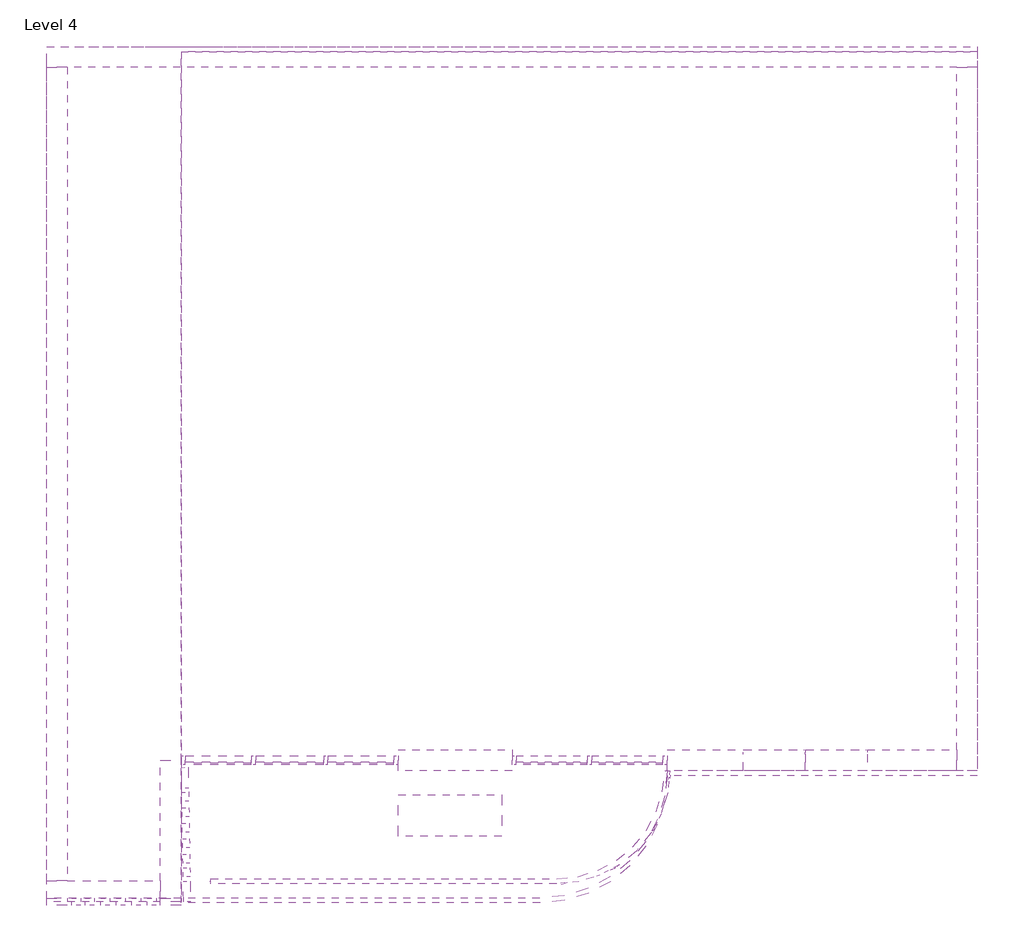
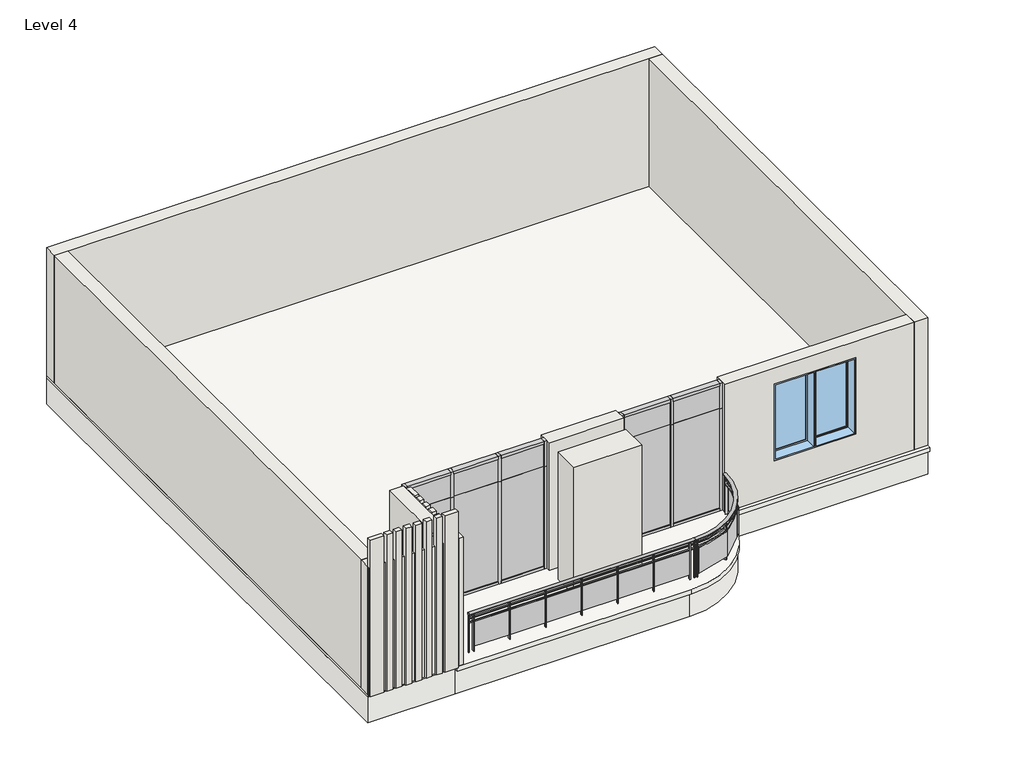
# One storey: 24 members, 24 walls, 10 plates, 3 slabs, 2 windows, 1 railing.
"""IFC4 building model written with IfcOpenShell, lengths in millimetres."""

from ifc_helpers import new_model, si_unit, point, frame, frame_2d, origin, place, context, project, spatial, polyline, circle_curve, ellipse_curve, trimmed, segment, composite_curve, outline, extrude, faceted_brep, transform, mapped, element, save
from ifc_brep_helpers import plane_surface, cylinder_surface, revolved_surface, extruded_surface, advanced_brep
from components import member_78934672, member_801a2072, member_cfcad22e, member_ee409385, member_47bfaf8a, member_f0fea5a5, member_6e77e263, system_panel_glazed_66ef8e2c, system_panel_glazed_30b75583, system_panel_glazed_387c9df4, system_panel_glazed_55a8196a, system_panel_glazed_9df4f396, system_panel_glazed_c1629c18, window_9a1f8bc2, window_c524ad49

model = new_model("IFC4")

# Units and contexts
model_context = context("Model", 3, world=origin())
ifc_project = project(units=[si_unit("LENGTHUNIT", "METRE", prefix="MILLI")], contexts=[model_context])

# Site, building, storey
site = spatial("IfcSite", under=ifc_project)
building = spatial("IfcBuilding", under=site)
storey = spatial("IfcBuildingStorey", under=building, Name="Level 4", Elevation=9144.0)

# Members
placement = place(None, origin())
member_shape = member_78934672(model_context)
element("IfcMember", 1, ObjectType="Rectangular Mullion : 2.5\" x 5\" rectangular", at=placement, inside=storey, context=model_context, shape_type="MappedRepresentation", body=[
    mapped(member_shape, transform((-10103.7104559, 977.728737, 11125.2), x_axis=(0.0, 0.0, -1.0), y_axis=(0.0, 1.0, 0.0), z_axis=(1.0, 0.0, 0.0))),
])
element("IfcMember", 2, ObjectType="Rectangular Mullion : 2.5\" x 5\" rectangular", at=placement, inside=storey, context=model_context, shape_type="MappedRepresentation", body=[
    mapped(member_shape, transform((-11214.9604559, 977.728737, 11125.2), x_axis=(0.0, 0.0, -1.0), y_axis=(0.0, 1.0, 0.0), z_axis=(1.0, 0.0, 0.0))),
])
element("IfcMember", 3, ObjectType="Rectangular Mullion : 2.5\" x 5\" rectangular", at=placement, inside=storey, context=model_context, shape_type="MappedRepresentation", body=[
    mapped(member_shape, transform((-12262.7104559, 977.728737, 14173.2), x_axis=(0.0, 0.0, 1.0), y_axis=(0.0, 1.0, 0.0), z_axis=(-1.0, 0.0, 0.0))),
])
element("IfcMember", 4, ObjectType="Rectangular Mullion : 2.5\" x 5\" rectangular", at=placement, inside=storey, context=model_context, shape_type="MappedRepresentation", body=[
    mapped(member_shape, transform((-11151.4604559, 977.728737, 14173.2), x_axis=(0.0, 0.0, 1.0), y_axis=(0.0, 1.0, 0.0), z_axis=(-1.0, 0.0, 0.0))),
])
member_2_shape = member_801a2072(model_context)
element("IfcMember", 5, ObjectType="Rectangular Mullion : 2.5\" x 5\" rectangular", at=placement, inside=storey, context=model_context, shape_type="MappedRepresentation", body=[
    mapped(member_2_shape, transform((-17139.5104559, 977.728737, 14173.2), x_axis=(0.0, 0.0, 1.0), y_axis=(0.0, 1.0, 0.0), z_axis=(-1.0, 0.0, 0.0))),
])
element("IfcMember", 6, ObjectType="Rectangular Mullion : 2.5\" x 5\" rectangular", at=placement, inside=storey, context=model_context, shape_type="MappedRepresentation", body=[
    mapped(member_2_shape, transform((-15037.6604559, 977.728737, 14173.2), x_axis=(0.0, 0.0, 1.0), y_axis=(0.0, 1.0, 0.0), z_axis=(-1.0, 0.0, 0.0))),
])
element("IfcMember", 7, ObjectType="Rectangular Mullion : 2.5\" x 5\" rectangular", at=placement, inside=storey, context=model_context, shape_type="MappedRepresentation", body=[
    mapped(member_2_shape, transform((-14066.1104559, 977.728737, 11125.2), x_axis=(0.0, 0.0, -1.0), y_axis=(0.0, 1.0, 0.0), z_axis=(1.0, 0.0, 0.0))),
])
element("IfcMember", 8, ObjectType="Rectangular Mullion : 2.5\" x 5\" rectangular", at=placement, inside=storey, context=model_context, shape_type="MappedRepresentation", body=[
    mapped(member_2_shape, transform((-16167.9604559, 977.728737, 11125.2), x_axis=(0.0, 0.0, -1.0), y_axis=(0.0, 1.0, 0.0), z_axis=(1.0, 0.0, 0.0))),
])
member_3_shape = member_cfcad22e(model_context)
element("IfcMember", 9, ObjectType="Rectangular Mullion : 2.5\" x 5\" rectangular", at=placement, inside=storey, context=model_context, shape_type="MappedRepresentation", body=[
    mapped(member_3_shape, transform((-15101.1604559, 977.728737, 11125.2), x_axis=(0.0, 0.0, -1.0), y_axis=(0.0, 1.0, 0.0), z_axis=(1.0, 0.0, 0.0))),
])
element("IfcMember", 10, ObjectType="Rectangular Mullion : 2.5\" x 5\" rectangular", at=placement, inside=storey, context=model_context, shape_type="MappedRepresentation", body=[
    mapped(member_3_shape, transform((-16104.4604559, 977.728737, 14173.2), x_axis=(0.0, 0.0, 1.0), y_axis=(0.0, 1.0, 0.0), z_axis=(-1.0, 0.0, 0.0))),
])
member_4_shape = member_ee409385(model_context)
element("IfcMember", 11, ObjectType="Rectangular Mullion : 2.5\" x 5\" rectangular", at=placement, inside=storey, context=model_context, shape_type="MappedRepresentation", body=[
    mapped(member_4_shape, transform((-12326.2104559, 977.728737, 11125.2), x_axis=(-1.0, 0.0, 0.0), y_axis=(0.0, 1.0, 0.0), z_axis=(0.0, 0.0, -1.0))),
])
element("IfcMember", 12, ObjectType="Rectangular Mullion : 2.5\" x 5\" rectangular", at=placement, inside=storey, context=model_context, shape_type="MappedRepresentation", body=[
    mapped(member_4_shape, transform((-17203.0104559, 977.728737, 11125.2), x_axis=(-1.0, 0.0, 0.0), y_axis=(0.0, 1.0, 0.0), z_axis=(0.0, 0.0, -1.0))),
])
member_5_shape = member_47bfaf8a(model_context)
element("IfcMember", 13, ObjectType="Rectangular Mullion : 2.5\" x 5\" rectangular", at=placement, inside=storey, context=model_context, shape_type="MappedRepresentation", body=[
    mapped(member_5_shape, transform((-12326.2104559, 977.728737, 13563.6), x_axis=(-1.0, 0.0, 0.0), y_axis=(0.0, 1.0, 0.0), z_axis=(0.0, 0.0, -1.0))),
])
element("IfcMember", 14, ObjectType="Rectangular Mullion : 2.5\" x 5\" rectangular", at=placement, inside=storey, context=model_context, shape_type="MappedRepresentation", body=[
    mapped(member_5_shape, transform((-17203.0104559, 977.728737, 13563.6), x_axis=(-1.0, 0.0, 0.0), y_axis=(0.0, 1.0, 0.0), z_axis=(0.0, 0.0, -1.0))),
])
member_6_shape = member_f0fea5a5(model_context)
element("IfcMember", 15, ObjectType="Rectangular Mullion : 2.5\" x 5\" rectangular", at=placement, inside=storey, context=model_context, shape_type="MappedRepresentation", body=[
    mapped(member_6_shape, transform((-11183.2104559, 977.728737, 11125.2), x_axis=(-1.0, 0.0, 0.0), y_axis=(0.0, 1.0, 0.0), z_axis=(0.0, 0.0, -1.0))),
])
element("IfcMember", 16, ObjectType="Rectangular Mullion : 2.5\" x 5\" rectangular", at=placement, inside=storey, context=model_context, shape_type="MappedRepresentation", body=[
    mapped(member_6_shape, transform((-15069.4104559, 977.728737, 11125.2), x_axis=(-1.0, 0.0, 0.0), y_axis=(0.0, 1.0, 0.0), z_axis=(0.0, 0.0, -1.0))),
])
element("IfcMember", 17, ObjectType="Rectangular Mullion : 2.5\" x 5\" rectangular", at=placement, inside=storey, context=model_context, shape_type="MappedRepresentation", body=[
    mapped(member_6_shape, transform((-16136.2104559, 977.728737, 11125.2), x_axis=(-1.0, 0.0, 0.0), y_axis=(0.0, 1.0, 0.0), z_axis=(0.0, 0.0, -1.0))),
])
member_7_shape = member_6e77e263(model_context)
element("IfcMember", 18, ObjectType="Rectangular Mullion : 2.5\" x 5\" rectangular", at=placement, inside=storey, context=model_context, shape_type="MappedRepresentation", body=[
    mapped(member_7_shape, transform((-11183.2104559, 977.728737, 13563.6), x_axis=(-1.0, 0.0, 0.0), y_axis=(0.0, 1.0, 0.0), z_axis=(0.0, 0.0, -1.0))),
])
element("IfcMember", 19, ObjectType="Rectangular Mullion : 2.5\" x 5\" rectangular", at=placement, inside=storey, context=model_context, shape_type="MappedRepresentation", body=[
    mapped(member_7_shape, transform((-15069.4104559, 977.728737, 13563.6), x_axis=(-1.0, 0.0, 0.0), y_axis=(0.0, 1.0, 0.0), z_axis=(0.0, 0.0, -1.0))),
])
element("IfcMember", 20, ObjectType="Rectangular Mullion : 2.5\" x 5\" rectangular", at=placement, inside=storey, context=model_context, shape_type="MappedRepresentation", body=[
    mapped(member_7_shape, transform((-16136.2104559, 977.728737, 13563.6), x_axis=(-1.0, 0.0, 0.0), y_axis=(0.0, 1.0, 0.0), z_axis=(0.0, 0.0, -1.0))),
])
element("IfcMember", 21, ObjectType="Rectangular Mullion : 2.5\" x 5\" rectangular", at=placement, inside=storey, context=model_context, shape_type="MappedRepresentation", body=[
    mapped(member_5_shape, transform((-10040.2104559, 977.728737, 14173.2), x_axis=(1.0, 0.0, 0.0), y_axis=(0.0, 1.0, 0.0), z_axis=(0.0, 0.0, 1.0))),
])
element("IfcMember", 22, ObjectType="Rectangular Mullion : 2.5\" x 5\" rectangular", at=placement, inside=storey, context=model_context, shape_type="MappedRepresentation", body=[
    mapped(member_5_shape, transform((-14002.6104559, 977.728737, 14173.2), x_axis=(1.0, 0.0, 0.0), y_axis=(0.0, 1.0, 0.0), z_axis=(0.0, 0.0, 1.0))),
])
element("IfcMember", 23, ObjectType="Rectangular Mullion : 2.5\" x 5\" rectangular", at=placement, inside=storey, context=model_context, shape_type="MappedRepresentation", body=[
    mapped(member_4_shape, transform((-10040.2104559, 977.728737, 13563.6), x_axis=(1.0, 0.0, 0.0), y_axis=(0.0, 1.0, 0.0), z_axis=(0.0, 0.0, 1.0))),
])
element("IfcMember", 24, ObjectType="Rectangular Mullion : 2.5\" x 5\" rectangular", at=placement, inside=storey, context=model_context, shape_type="MappedRepresentation", body=[
    mapped(member_4_shape, transform((-14002.6104559, 977.728737, 13563.6), x_axis=(1.0, 0.0, 0.0), y_axis=(0.0, 1.0, 0.0), z_axis=(0.0, 0.0, 1.0))),
])

# Plates
system_panel_glazed_shape = system_panel_glazed_66ef8e2c(model_context)
element("IfcPlate", 25, ObjectType="System Panel : Glazed", at=placement, inside=storey, context=model_context, shape_type="MappedRepresentation", body=[
    mapped(system_panel_glazed_shape, transform((-10627.5854559, 977.728737, 11188.7), x_axis=(-1.0, 0.0, 0.0), y_axis=(0.0, -1.0, 0.0), z_axis=(0.0, 0.0, 1.0))),
])
element("IfcPlate", 26, ObjectType="System Panel : Glazed", at=placement, inside=storey, context=model_context, shape_type="MappedRepresentation", body=[
    mapped(system_panel_glazed_shape, transform((-11738.8354559, 977.728737, 11188.7), x_axis=(-1.0, 0.0, 0.0), y_axis=(0.0, -1.0, 0.0), z_axis=(0.0, 0.0, 1.0))),
])
system_panel_glazed_2_shape = system_panel_glazed_30b75583(model_context)
element("IfcPlate", 27, ObjectType="System Panel : Glazed", at=placement, inside=storey, context=model_context, shape_type="MappedRepresentation", body=[
    mapped(system_panel_glazed_2_shape, transform((-10627.5854559, 977.728737, 13563.6), x_axis=(-1.0, 0.0, 0.0), y_axis=(0.0, -1.0, 0.0), z_axis=(0.0, 0.0, 1.0))),
])
element("IfcPlate", 28, ObjectType="System Panel : Glazed", at=placement, inside=storey, context=model_context, shape_type="MappedRepresentation", body=[
    mapped(system_panel_glazed_2_shape, transform((-11738.8354559, 977.728737, 13563.6), x_axis=(-1.0, 0.0, 0.0), y_axis=(0.0, -1.0, 0.0), z_axis=(0.0, 0.0, 1.0))),
])
system_panel_glazed_3_shape = system_panel_glazed_387c9df4(model_context)
element("IfcPlate", 29, ObjectType="System Panel : Glazed", at=placement, inside=storey, context=model_context, shape_type="MappedRepresentation", body=[
    mapped(system_panel_glazed_3_shape, transform((-14551.8854559, 977.728737, 11188.7), x_axis=(-1.0, 0.0, 0.0), y_axis=(0.0, -1.0, 0.0), z_axis=(0.0, 0.0, 1.0))),
])
element("IfcPlate", 30, ObjectType="System Panel : Glazed", at=placement, inside=storey, context=model_context, shape_type="MappedRepresentation", body=[
    mapped(system_panel_glazed_3_shape, transform((-16653.7354559, 977.728737, 11188.7), x_axis=(-1.0, 0.0, 0.0), y_axis=(0.0, -1.0, 0.0), z_axis=(0.0, 0.0, 1.0))),
])
system_panel_glazed_4_shape = system_panel_glazed_55a8196a(model_context)
element("IfcPlate", 31, ObjectType="System Panel : Glazed", at=placement, inside=storey, context=model_context, shape_type="MappedRepresentation", body=[
    mapped(system_panel_glazed_4_shape, transform((-14551.8854559, 977.728737, 13563.6), x_axis=(-1.0, 0.0, 0.0), y_axis=(0.0, -1.0, 0.0), z_axis=(0.0, 0.0, 1.0))),
])
element("IfcPlate", 32, ObjectType="System Panel : Glazed", at=placement, inside=storey, context=model_context, shape_type="MappedRepresentation", body=[
    mapped(system_panel_glazed_4_shape, transform((-16653.7354559, 977.728737, 13563.6), x_axis=(-1.0, 0.0, 0.0), y_axis=(0.0, -1.0, 0.0), z_axis=(0.0, 0.0, 1.0))),
])
system_panel_glazed_5_shape = system_panel_glazed_9df4f396(model_context)
element("IfcPlate", 33, ObjectType="System Panel : Glazed", at=placement, inside=storey, context=model_context, shape_type="MappedRepresentation", body=[
    mapped(system_panel_glazed_5_shape, transform((-15602.8104559, 977.728737, 11188.7), x_axis=(-1.0, 0.0, 0.0), y_axis=(0.0, -1.0, 0.0), z_axis=(0.0, 0.0, 1.0))),
])
system_panel_glazed_6_shape = system_panel_glazed_c1629c18(model_context)
element("IfcPlate", 34, ObjectType="System Panel : Glazed", at=placement, inside=storey, context=model_context, shape_type="MappedRepresentation", body=[
    mapped(system_panel_glazed_6_shape, transform((-15602.8104559, 977.728737, 13563.6), x_axis=(-1.0, 0.0, 0.0), y_axis=(0.0, -1.0, 0.0), z_axis=(0.0, 0.0, 1.0))),
])

# Railing
element("IfcRailing", 35, ObjectType="Glass Panel - Bottom Fill", at=placement, inside=storey, context=model_context, shape_type="SolidModel", body=[
    advanced_brep(
    [(-16762.7787181, -765.7171954, 12039.6), (-16762.7787181, -841.9171954, 12039.6), (-11669.3563882, -765.7171954, 12039.6), (-11669.3563882, -841.9171954, 12039.6), (-10002.1104559, 825.328737, 12039.6), (-10078.3104559, 825.328737, 12039.6)],
    [
        (0, 1, ellipse_curve(frame((-16762.7787181, -803.8171954, 12039.6), z_axis=(-1.0, 0.0, 0.0), x_axis=(0.0, -1.0, 0.0)), 38.1, 28.575)),
        (1, 0, ellipse_curve(frame((-16762.7787181, -803.8171954, 12039.6), z_axis=(-1.0, 0.0, 0.0), x_axis=(0.0, -1.0, 0.0)), 38.1, 28.575)),
        (0, 2),
        (2, 3, ellipse_curve(frame((-11669.3563882, -803.8171954, 12039.6), z_axis=(-1.0, 0.0, 0.0), x_axis=(0.0, -1.0, 0.0)), 38.1, 28.575)),
        (3, 1),
        (3, 2, ellipse_curve(frame((-11669.3563882, -803.8171954, 12039.6), z_axis=(-1.0, 0.0, 0.0), x_axis=(0.0, -1.0, 0.0)), 38.1, 28.575)),
        (4, 3, circle_curve(frame((-11669.3563882, 825.328737, 12039.6), z_axis=(0.0, 0.0, -1.0), x_axis=(0.0, -1.0, 0.0)), 1667.2459324)),
        (2, 5, circle_curve(frame((-11669.3563882, 825.328737, 12039.6), z_axis=(0.0, 0.0, 1.0), x_axis=(0.0, -1.0, 0.0)), 1591.0459324)),
        (5, 4, ellipse_curve(frame((-10040.2104559, 825.328737, 12039.6), z_axis=(0.0, -1.0, 0.0), x_axis=(1.0, 0.0, 0.0)), 38.1, 28.575)),
        (4, 5, ellipse_curve(frame((-10040.2104559, 825.328737, 12039.6), z_axis=(0.0, -1.0, 0.0), x_axis=(1.0, 0.0, 0.0)), 38.1, 28.575)),
    ],
    [
        plane_surface(frame((-16762.7787181, -803.8171954, 12039.6), z_axis=(-1.0, 0.0, 0.0), x_axis=(0.0, 1.0, 0.0))),
        extruded_surface(trimmed(ellipse_curve(frame((-11669.3563882, -803.8171954, 12039.6), z_axis=(-1.0, 0.0, 0.0), x_axis=(0.0, -1.0, 0.0)), 38.1, 28.575), [point((-11669.3563882, -765.7171954, 12039.6))], [point((-11669.3563882, -841.9171954, 12039.6))], True, "CARTESIAN"), (-5093.422329899999, 0.0, 0.0), 5093.422329899999),
        extruded_surface(trimmed(ellipse_curve(frame((-11669.3563882, -803.8171954, 12039.6), z_axis=(-1.0, 0.0, 0.0), x_axis=(0.0, -1.0, 0.0)), 38.1, 28.575), [point((-11669.3563882, -841.9171954, 12039.6))], [point((-11669.3563882, -765.7171954, 12039.6))], True, "CARTESIAN"), (-5093.422329899999, 0.0, 0.0), 5093.422329899999),
        revolved_surface(trimmed(ellipse_curve(frame((-11669.3563882, -803.8171954, 12039.6), z_axis=(-1.0, 0.0, 0.0), x_axis=(0.0, -1.0, 0.0)), 38.1, 28.575), [point((-11669.3563882, -765.7171954, 12039.6))], [point((-11669.3563882, -841.9171954, 12039.6))], True, "CARTESIAN"), (-11669.3563882, 825.328737, 12039.6), (0.0, 0.0, 1.0)),
        revolved_surface(trimmed(ellipse_curve(frame((-11669.3563882, -803.8171954, 12039.6), z_axis=(-1.0, 0.0, 0.0), x_axis=(0.0, -1.0, 0.0)), 38.1, 28.575), [point((-11669.3563882, -841.9171954, 12039.6))], [point((-11669.3563882, -765.7171954, 12039.6))], True, "CARTESIAN"), (-11669.3563882, 825.328737, 12039.6), (0.0, 0.0, 1.0)),
        plane_surface(frame((-10040.2104559, 825.328737, 12039.6), z_axis=(0.0, 1.0, 0.0), x_axis=(0.0, 0.0, 1.0))),
    ],
    [
        (0, [[1, 2]]),
        (1, [[-1, 3, 4, 5]]),
        (2, [[-2, -5, 6, -3]]),
        (3, [[7, -4, 8, 9]]),
        (4, [[-8, -6, -7, 10]]),
        (5, [[-10, -9]]),
    ],
),
    advanced_brep(
    [(-16762.7787181, -816.5171954, 11950.7), (-16762.7787181, -791.1171954, 11950.7), (-16762.7787181, -791.1171954, 11925.3), (-16762.7787181, -816.5171954, 11925.3), (-11669.3563882, -816.5171954, 11950.7), (-11669.3563882, -791.1171954, 11950.7), (-11669.3563882, -791.1171954, 11925.3), (-11669.3563882, -816.5171954, 11925.3), (-10052.9104559, 825.328737, 11950.7), (-10027.5104559, 825.328737, 11950.7), (-10052.9104559, 825.328737, 11925.3), (-10027.5104559, 825.328737, 11925.3)],
    [
        (0, 1),
        (1, 2),
        (2, 3),
        (3, 0),
        (0, 4),
        (4, 5),
        (5, 1),
        (5, 6),
        (6, 2),
        (6, 7),
        (7, 3),
        (7, 4),
        (8, 5, circle_curve(frame((-11669.3563882, 825.328737, 11950.7), z_axis=(0.0, 0.0, -1.0), x_axis=(0.0, -1.0, 0.0)), 1616.4459324)),
        (4, 9, circle_curve(frame((-11669.3563882, 825.328737, 11950.7), z_axis=(0.0, 0.0, 1.0), x_axis=(0.0, -1.0, 0.0)), 1641.8459324)),
        (9, 8),
        (10, 6, circle_curve(frame((-11669.3563882, 825.328737, 11925.3), z_axis=(0.0, 0.0, -1.0), x_axis=(0.0, -1.0, 0.0)), 1616.4459324)),
        (8, 10),
        (11, 7, circle_curve(frame((-11669.3563882, 825.328737, 11925.3), z_axis=(0.0, 0.0, -1.0), x_axis=(0.0, -1.0, 0.0)), 1641.8459324)),
        (10, 11),
        (11, 9),
    ],
    [
        plane_surface(frame((-16762.7787181, -803.8171954, 11938.0), z_axis=(-1.0, 0.0, 0.0), x_axis=(0.0, 1.0, 0.0))),
        plane_surface(frame((-16762.7787181, -816.5171954, 11950.7), z_axis=(0.0, 0.0, 1.0), x_axis=(1.0, 0.0, 0.0))),
        plane_surface(frame((-16762.7787181, -791.1171954, 11950.7), z_axis=(0.0, 1.0, 0.0), x_axis=(1.0, 0.0, 0.0))),
        plane_surface(frame((-16762.7787181, -791.1171954, 11925.3), z_axis=(0.0, 0.0, -1.0), x_axis=(1.0, 0.0, 0.0))),
        plane_surface(frame((-16762.7787181, -816.5171954, 11925.3), z_axis=(0.0, -1.0, 0.0), x_axis=(1.0, 0.0, 0.0))),
        plane_surface(frame((-11669.3563882, 825.328737, 11950.7), z_axis=(0.0, 0.0, 1.0), x_axis=(0.0, -1.0, 0.0))),
        revolved_surface(polyline([(-11669.3563882, -791.1171953999999, 11950.7), (-11669.3563882, -791.1171953999999, 11925.3)]), (-11669.3563882, 825.328737, 11938.0), (0.0, 0.0, 1.0)),
        plane_surface(frame((-11669.3563882, 825.328737, 11925.3), z_axis=(0.0, 0.0, -1.0), x_axis=(0.0, -1.0, 0.0))),
        cylinder_surface(frame((-11669.3563882, 825.328737, 11938.0), z_axis=(0.0, 0.0, 1.0), x_axis=(0.0, -1.0, 0.0)), 1641.8459324),
        plane_surface(frame((-10040.2104559, 825.328737, 11938.0), z_axis=(0.0, 1.0, 0.0), x_axis=(0.0, 0.0, 1.0))),
    ],
    [
        (0, [[1, 2, 3, 4]]),
        (1, [[-1, 5, 6, 7]]),
        (2, [[-2, -7, 8, 9]]),
        (3, [[-3, -9, 10, 11]]),
        (4, [[-4, -11, 12, -5]]),
        (5, [[13, -6, 14, 15]]),
        (6, [[16, -8, -13, 17]]),
        (7, [[18, -10, -16, 19]]),
        (8, [[-14, -12, -18, 20]]),
        (9, [[-20, -19, -17, -15]]),
    ],
),
    advanced_brep(
    [(-16762.7787181, -816.5171954, 11849.1), (-16762.7787181, -791.1171954, 11849.1), (-16762.7787181, -791.1171954, 11823.7), (-16762.7787181, -816.5171954, 11823.7), (-11669.3563882, -816.5171954, 11849.1), (-11669.3563882, -791.1171954, 11849.1), (-11669.3563882, -791.1171954, 11823.7), (-11669.3563882, -816.5171954, 11823.7), (-10052.9104559, 825.328737, 11849.1), (-10027.5104559, 825.328737, 11849.1), (-10052.9104559, 825.328737, 11823.7), (-10027.5104559, 825.328737, 11823.7)],
    [
        (0, 1),
        (1, 2),
        (2, 3),
        (3, 0),
        (0, 4),
        (4, 5),
        (5, 1),
        (5, 6),
        (6, 2),
        (6, 7),
        (7, 3),
        (7, 4),
        (8, 5, circle_curve(frame((-11669.3563882, 825.328737, 11849.1), z_axis=(0.0, 0.0, -1.0), x_axis=(0.0, -1.0, 0.0)), 1616.4459324)),
        (4, 9, circle_curve(frame((-11669.3563882, 825.328737, 11849.1), z_axis=(0.0, 0.0, 1.0), x_axis=(0.0, -1.0, 0.0)), 1641.8459324)),
        (9, 8),
        (10, 6, circle_curve(frame((-11669.3563882, 825.328737, 11823.7), z_axis=(0.0, 0.0, -1.0), x_axis=(0.0, -1.0, 0.0)), 1616.4459324)),
        (8, 10),
        (11, 7, circle_curve(frame((-11669.3563882, 825.328737, 11823.7), z_axis=(0.0, 0.0, -1.0), x_axis=(0.0, -1.0, 0.0)), 1641.8459324)),
        (10, 11),
        (11, 9),
    ],
    [
        plane_surface(frame((-16762.7787181, -803.8171954, 11836.4), z_axis=(-1.0, 0.0, 0.0), x_axis=(0.0, 1.0, 0.0))),
        plane_surface(frame((-16762.7787181, -816.5171954, 11849.1), z_axis=(0.0, 0.0, 1.0), x_axis=(1.0, 0.0, 0.0))),
        plane_surface(frame((-16762.7787181, -791.1171954, 11849.1), z_axis=(0.0, 1.0, 0.0), x_axis=(1.0, 0.0, 0.0))),
        plane_surface(frame((-16762.7787181, -791.1171954, 11823.7), z_axis=(0.0, 0.0, -1.0), x_axis=(1.0, 0.0, 0.0))),
        plane_surface(frame((-16762.7787181, -816.5171954, 11823.7), z_axis=(0.0, -1.0, 0.0), x_axis=(1.0, 0.0, 0.0))),
        plane_surface(frame((-11669.3563882, 825.328737, 11849.1), z_axis=(0.0, 0.0, 1.0), x_axis=(0.0, -1.0, 0.0))),
        revolved_surface(polyline([(-11669.3563882, -791.1171953999999, 11849.1), (-11669.3563882, -791.1171953999999, 11823.7)]), (-11669.3563882, 825.328737, 11836.4), (0.0, 0.0, 1.0)),
        plane_surface(frame((-11669.3563882, 825.328737, 11823.7), z_axis=(0.0, 0.0, -1.0), x_axis=(0.0, -1.0, 0.0))),
        cylinder_surface(frame((-11669.3563882, 825.328737, 11836.4), z_axis=(0.0, 0.0, 1.0), x_axis=(0.0, -1.0, 0.0)), 1641.8459324),
        plane_surface(frame((-10040.2104559, 825.328737, 11836.4), z_axis=(0.0, 1.0, 0.0), x_axis=(0.0, 0.0, 1.0))),
    ],
    [
        (0, [[1, 2, 3, 4]]),
        (1, [[-1, 5, 6, 7]]),
        (2, [[-2, -7, 8, 9]]),
        (3, [[-3, -9, 10, 11]]),
        (4, [[-4, -11, 12, -5]]),
        (5, [[13, -6, 14, 15]]),
        (6, [[16, -8, -13, 17]]),
        (7, [[18, -10, -16, 19]]),
        (8, [[-14, -12, -18, 20]]),
        (9, [[-20, -19, -17, -15]]),
    ],
),
    extrude(outline(polyline([(-10016.1798264, 757.7282919), (-10066.9450003, 759.6090156), (-10066.4748193, 772.3003091), (-10015.7096455, 770.4195853), (-10016.1798264, 757.7282919)])), frame((0.0, 0.0, 11125.2), z_axis=(0.0, 0.0, 1.0), x_axis=(1.0, 0.0, 0.0)), (0.0, 0.0, 1.0), 885.6788223),
    extrude(outline(polyline([(-10227.7208829, -23.0307141), (-9998.0369146, 756.6417265), (-9991.9457237, 754.8473205), (-10221.629692, -24.8251201), (-10227.7208829, -23.0307141)])), frame((0.0, 0.0, 11226.8), z_axis=(0.0, 0.0, 1.0), x_axis=(1.0, 0.0, 0.0)), (0.0, 0.0, 1.0), 596.9),
    extrude(outline(polyline([(-10250.0405804, -25.0271899), (-10293.7178017, 0.9139036), (-10287.2325284, 11.8332089), (-10243.555307, -14.1078846), (-10250.0405804, -25.0271899)])), frame((0.0, 0.0, 11125.2), z_axis=(0.0, 0.0, 1.0), x_axis=(1.0, 0.0, 0.0)), (0.0, 0.0, 1.0), 885.6788223),
    extrude(outline(polyline([(-10809.3655016, -609.3985414), (-10234.6291099, -34.6621497), (-10230.1389818, -39.1522777), (-10804.8753736, -613.8886695), (-10809.3655016, -609.3985414)])), frame((0.0, 0.0, 11226.8), z_axis=(0.0, 0.0, 1.0), x_axis=(1.0, 0.0, 0.0)), (0.0, 0.0, 1.0), 596.9),
    extrude(outline(polyline([(-10829.9197667, -600.4723443), (-10855.8608602, -556.7951229), (-10844.9415549, -550.3098495), (-10819.0004614, -593.9870709), (-10829.9197667, -600.4723443)])), frame((0.0, 0.0, 11125.2), z_axis=(0.0, 0.0, 1.0), x_axis=(1.0, 0.0, 0.0)), (0.0, 0.0, 1.0), 885.6788223),
    extrude(outline(polyline([(-11600.6693778, -845.9907367), (-10820.9969372, -616.3067684), (-10819.2025312, -622.3979593), (-11598.8749718, -852.0819276), (-11600.6693778, -845.9907367)])), frame((0.0, 0.0, 11226.8), z_axis=(0.0, 0.0, 1.0), x_axis=(1.0, 0.0, 0.0)), (0.0, 0.0, 1.0), 596.9),
    extrude(outline(polyline([(-11614.4472366, -828.3180058), (-11616.3279603, -777.552832), (-11603.6366669, -777.082651), (-11601.7559432, -827.8478249), (-11614.4472366, -828.3180058)])), frame((0.0, 0.0, 11125.2), z_axis=(0.0, 0.0, 1.0), x_axis=(1.0, 0.0, 0.0)), (0.0, 0.0, 1.0), 885.6788223),
    extrude(outline(polyline([(-11784.0175532, -829.2171954), (-11784.0175532, -778.4171954), (-11771.3175532, -778.4171954), (-11771.3175532, -829.2171954), (-11784.0175532, -829.2171954)])), frame((0.0, 0.0, 11125.2), z_axis=(0.0, 0.0, 1.0), x_axis=(1.0, 0.0, 0.0)), (0.0, 0.0, 1.0), 885.6788223),
    extrude(outline(polyline([(-12590.4675532, -797.2820384), (-11777.6675532, -797.2820384), (-11777.6675532, -803.6320384), (-12590.4675532, -803.6320384), (-12590.4675532, -797.2820384)])), frame((0.0, 0.0, 11226.8), z_axis=(0.0, 0.0, 1.0), x_axis=(1.0, 0.0, 0.0)), (0.0, 0.0, 1.0), 596.9),
    extrude(outline(polyline([(-12596.8175532, -829.2171954), (-12596.8175532, -778.4171954), (-12584.1175532, -778.4171954), (-12584.1175532, -829.2171954), (-12596.8175532, -829.2171954)])), frame((0.0, 0.0, 11125.2), z_axis=(0.0, 0.0, 1.0), x_axis=(1.0, 0.0, 0.0)), (0.0, 0.0, 1.0), 885.6788223),
    extrude(outline(polyline([(-13403.2675532, -797.2820384), (-12590.4675532, -797.2820384), (-12590.4675532, -803.6320384), (-13403.2675532, -803.6320384), (-13403.2675532, -797.2820384)])), frame((0.0, 0.0, 11226.8), z_axis=(0.0, 0.0, 1.0), x_axis=(1.0, 0.0, 0.0)), (0.0, 0.0, 1.0), 596.9),
    extrude(outline(polyline([(-13409.6175532, -829.2171954), (-13409.6175532, -778.4171954), (-13396.9175532, -778.4171954), (-13396.9175532, -829.2171954), (-13409.6175532, -829.2171954)])), frame((0.0, 0.0, 11125.2), z_axis=(0.0, 0.0, 1.0), x_axis=(1.0, 0.0, 0.0)), (0.0, 0.0, 1.0), 885.6788223),
    extrude(outline(polyline([(-14216.0675532, -797.2820384), (-13403.2675532, -797.2820384), (-13403.2675532, -803.6320384), (-14216.0675532, -803.6320384), (-14216.0675532, -797.2820384)])), frame((0.0, 0.0, 11226.8), z_axis=(0.0, 0.0, 1.0), x_axis=(1.0, 0.0, 0.0)), (0.0, 0.0, 1.0), 596.9),
    extrude(outline(polyline([(-14222.4175532, -829.2171954), (-14222.4175532, -778.4171954), (-14209.7175532, -778.4171954), (-14209.7175532, -829.2171954), (-14222.4175532, -829.2171954)])), frame((0.0, 0.0, 11125.2), z_axis=(0.0, 0.0, 1.0), x_axis=(1.0, 0.0, 0.0)), (0.0, 0.0, 1.0), 885.6788223),
    extrude(outline(polyline([(-15028.8675532, -797.2820384), (-14216.0675532, -797.2820384), (-14216.0675532, -803.6320384), (-15028.8675532, -803.6320384), (-15028.8675532, -797.2820384)])), frame((0.0, 0.0, 11226.8), z_axis=(0.0, 0.0, 1.0), x_axis=(1.0, 0.0, 0.0)), (0.0, 0.0, 1.0), 596.9),
    extrude(outline(polyline([(-15035.2175532, -829.2171954), (-15035.2175532, -778.4171954), (-15022.5175532, -778.4171954), (-15022.5175532, -829.2171954), (-15035.2175532, -829.2171954)])), frame((0.0, 0.0, 11125.2), z_axis=(0.0, 0.0, 1.0), x_axis=(1.0, 0.0, 0.0)), (0.0, 0.0, 1.0), 885.6788223),
    extrude(outline(polyline([(-15841.6675532, -797.2820384), (-15028.8675532, -797.2820384), (-15028.8675532, -803.6320384), (-15841.6675532, -803.6320384), (-15841.6675532, -797.2820384)])), frame((0.0, 0.0, 11226.8), z_axis=(0.0, 0.0, 1.0), x_axis=(1.0, 0.0, 0.0)), (0.0, 0.0, 1.0), 596.9),
    extrude(outline(polyline([(-15848.0175532, -829.2171954), (-15848.0175532, -778.4171954), (-15835.3175532, -778.4171954), (-15835.3175532, -829.2171954), (-15848.0175532, -829.2171954)])), frame((0.0, 0.0, 11125.2), z_axis=(0.0, 0.0, 1.0), x_axis=(1.0, 0.0, 0.0)), (0.0, 0.0, 1.0), 885.6788223),
    extrude(outline(polyline([(-16654.4675532, -797.2820384), (-15841.6675532, -797.2820384), (-15841.6675532, -803.6320384), (-16654.4675532, -803.6320384), (-16654.4675532, -797.2820384)])), frame((0.0, 0.0, 11226.8), z_axis=(0.0, 0.0, 1.0), x_axis=(1.0, 0.0, 0.0)), (0.0, 0.0, 1.0), 596.9),
    extrude(outline(polyline([(-16660.8175532, -829.2171954), (-16660.8175532, -778.4171954), (-16648.1175532, -778.4171954), (-16648.1175532, -829.2171954), (-16660.8175532, -829.2171954)])), frame((0.0, 0.0, 11125.2), z_axis=(0.0, 0.0, 1.0), x_axis=(1.0, 0.0, 0.0)), (0.0, 0.0, 1.0), 885.6788223),
    extrude(outline(polyline([(-11678.8813882, -813.3421954), (-11678.8813882, -794.2921954), (-11659.8313882, -794.2921954), (-11659.8313882, -813.3421954), (-11678.8813882, -813.3421954)])), frame((0.0, 0.0, 11125.2), z_axis=(0.0, 0.0, 1.0), x_axis=(1.0, 0.0, 0.0)), (0.0, 0.0, 1.0), 885.6788223),
    extrude(outline(polyline([(-10030.7071308, 812.610194), (-10049.7570946, 812.6473201), (-10049.7199686, 831.6972839), (-10030.6700048, 831.6601579), (-10030.7071308, 812.610194)])), frame((0.0, 0.0, 11125.2), z_axis=(0.0, 0.0, 1.0), x_axis=(1.0, 0.0, 0.0)), (0.0, 0.0, 1.0), 885.6788223),
    extrude(outline(polyline([(-16769.1287181, -813.3421954), (-16769.1287181, -794.2921954), (-16750.0787181, -794.2921954), (-16750.0787181, -813.3421954), (-16769.1287181, -813.3421954)])), frame((0.0, 0.0, 11125.2), z_axis=(0.0, 0.0, 1.0), x_axis=(1.0, 0.0, 0.0)), (0.0, 0.0, 1.0), 885.6788223),
])

# Slabs
element("IfcSlab", 36, ObjectType="Generic - 4\"", at=placement, inside=storey, context=model_context, shape_type="SweptSolid", body=[
    extrude(outline(polyline([(-17203.0104559, 11493.328737), (-5468.2104559, 11493.328737), (-5468.2104559, 11417.128737), (-17203.0104559, 11417.128737), (-17203.0104559, -1054.271263), (-19184.2104559, -1054.271263), (-19184.2104559, 11493.328737), (-17203.0104559, 11493.328737)])), frame((0.0, 0.0, 11023.6), z_axis=(0.0, 0.0, 1.0), x_axis=(1.0, 0.0, 0.0)), (0.0, 0.0, 1.0), 101.6),
])
element("IfcSlab", 37, ObjectType="LW Concrete on Metal Deck", at=placement, inside=storey, context=model_context, shape_type="SweptSolid", body=[
    extrude(outline(composite_curve([segment(polyline([(-5468.2104559, 11417.128737), (-5468.2104559, 749.128737), (-10040.2104559, 749.128737)]), True, "CONTINUOUS"), segment(trimmed(circle_curve(frame_2d((-11913.4604559, 749.128737)), 1873.25), [point((-10040.2104559, 749.128737))], [point((-11913.4604559, -1124.121263))], False, "CARTESIAN"), True, "CONTINUOUS"), segment(polyline([(-11913.4604559, -1124.121263), (-17203.0104559, -1124.121263), (-17203.0104559, 11417.128737), (-5468.2104559, 11417.128737)]), True, "CONTINUOUS")], self_intersect=False)), frame((0.0, 0.0, 11020.425), z_axis=(0.0, 0.0, 1.0), x_axis=(1.0, 0.0, 0.0)), (0.0, 0.0, 1.0), 104.775),
])
element("IfcSlab", 38, ObjectType="wall design 2", at=placement, inside=storey, context=model_context, shape_type="SweptSolid", body=[
    extrude(outline(composite_curve([segment(polyline([(-5468.2104559, 11493.328737), (-5468.2104559, 825.328737), (-10040.2104559, 825.328737)]), True, "CONTINUOUS"), segment(trimmed(circle_curve(frame_2d((-11919.8104559, 825.328737)), 1879.6), [point((-10040.2104559, 825.328737))], [point((-11919.8104559, -1054.271263))], False, "CARTESIAN"), True, "CONTINUOUS"), segment(polyline([(-11919.8104559, -1054.271263), (-17203.0104559, -1054.271263), (-19184.2104559, -1054.271263), (-19184.2104559, 11493.328737), (-5468.2104559, 11493.328737)]), True, "CONTINUOUS")], self_intersect=False)), frame((0.0, 0.0, 10439.4), z_axis=(0.0, 0.0, 1.0), x_axis=(1.0, 0.0, 0.0)), (0.0, 0.0, 1.0), 609.6),
])

# Walls
element("IfcWall", 39, ObjectType="Generic - 12\" 2", at=placement, inside=storey, context=model_context, shape_type="Brep", body=[
    faceted_brep([(-19184.2104559, 11188.528737, 11125.2), (-18879.4104559, 11188.528737, 11125.2), (-5773.0104559, 11188.528737, 11125.2), (-5468.2104559, 11188.528737, 11125.2), (-5468.2104559, 11188.528737, 14173.2), (-5773.0104559, 11188.528737, 14173.2), (-18879.4104559, 11188.528737, 14173.2), (-19184.2104559, 11188.528737, 14173.2), (-19184.2104559, 11493.328737, 11125.2), (-19184.2104559, 11493.328737, 14173.2), (-5468.2104559, 11493.328737, 14173.2), (-5468.2104559, 11493.328737, 11125.2)], [[[0, 1, 2, 3, 4, 5, 6, 7]], [[8, 9, 10, 11]], [[3, 2, 1, 0, 8, 11]], [[7, 6, 5, 4, 10, 9]], [[4, 3, 11, 10]], [[0, 7, 9, 8]]]),
])
element("IfcWall", 40, ObjectType="Generic - 12\" 2", at=placement, inside=storey, context=model_context, shape_type="Brep", body=[
    faceted_brep([(-5773.0104559, 11188.528737, 11125.2), (-5773.0104559, 1130.128737, 11125.2), (-5773.0104559, 825.328737, 11125.2), (-5773.0104559, 825.328737, 14173.2), (-5773.0104559, 1130.128737, 14173.2), (-5773.0104559, 11188.528737, 14173.2), (-5468.2104559, 11188.528737, 11125.2), (-5468.2104559, 11188.528737, 14173.2), (-5468.2104559, 825.328737, 14173.2), (-5468.2104559, 825.328737, 11125.2)], [[[0, 1, 2, 3, 4, 5]], [[6, 7, 8, 9]], [[2, 1, 0, 6, 9]], [[5, 4, 3, 8, 7]], [[0, 5, 7, 6]], [[3, 2, 9, 8]]]),
])
element("IfcWall", 41, ObjectType="Generic - 12\" 2", at=placement, inside=storey, context=model_context, shape_type="SweptSolid", body=[
    extrude(outline(polyline([(11125.2, -10040.2104559), (11125.2, -5773.0104559), (14173.2, -5773.0104559), (14173.2, -10040.2104559), (11125.2, -10040.2104559)]), holes=[polyline([(11963.4, -8922.6104559), (13792.2, -8922.6104559), (13792.2, -8008.2104559), (13790.0260244, -8008.2104559), (13790.0260244, -7093.8104559), (11961.2260244, -7093.8104559), (11961.2260244, -8008.2104559), (11963.4, -8008.2104559), (11963.4, -8922.6104559)])]), frame((0.0, 825.328737, 0.0), z_axis=(0.0, 1.0, 0.0), x_axis=(0.0, 0.0, 1.0)), (0.0, 0.0, 1.0), 304.8),
])
element("IfcWall", 42, ObjectType="Generic - 12\" 2", at=placement, inside=storey, context=model_context, shape_type="Brep", body=[
    faceted_brep([(-17507.8104559, 977.728737, 11125.2), (-17507.8104559, -800.271263, 11125.2), (-17507.8104559, -1105.071263, 11125.2), (-17507.8104559, -1105.071263, 14173.2), (-17507.8104559, -800.271263, 14173.2), (-17507.8104559, 977.728737, 14173.2), (-17203.0104559, 977.728737, 11125.2), (-17203.0104559, 977.728737, 14173.2), (-17203.0104559, -1105.071263, 14173.2), (-17203.0104559, -1105.071263, 11125.2)], [[[0, 1, 2, 3, 4, 5]], [[6, 7, 8, 9]], [[2, 1, 0, 6, 9]], [[5, 4, 3, 8, 7]], [[0, 5, 7, 6]], [[3, 2, 9, 8]]]),
])
element("IfcWall", 43, ObjectType="Generic - 12\" 2", at=placement, inside=storey, context=model_context, shape_type="Brep", body=[
    faceted_brep([(-17507.8104559, -800.271263, 11125.2), (-18879.4104559, -800.271263, 11125.2), (-19184.2104559, -800.271263, 11125.2), (-19184.2104559, -800.271263, 14173.2), (-18879.4104559, -800.271263, 14173.2), (-17507.8104559, -800.271263, 14173.2), (-17507.8104559, -1105.071263, 11125.2), (-17507.8104559, -1105.071263, 14173.2), (-19184.2104559, -1105.071263, 14173.2), (-19184.2104559, -1105.071263, 11125.2)], [[[0, 1, 2, 3, 4, 5]], [[6, 7, 8, 9]], [[2, 1, 0, 6, 9]], [[5, 4, 3, 8, 7]], [[0, 5, 7, 6]], [[3, 2, 9, 8]]]),
])
element("IfcWall", 44, ObjectType="Generic - 12\" 2", at=placement, inside=storey, context=model_context, shape_type="SweptSolid", body=[
    extrude(outline(polyline([(-18879.4104559, 11188.528737), (-18879.4104559, -800.271263), (-19184.2104559, -800.271263), (-19184.2104559, 11188.528737), (-18879.4104559, 11188.528737)])), frame((0.0, 0.0, 11125.2), z_axis=(0.0, 0.0, 1.0), x_axis=(1.0, 0.0, 0.0)), (0.0, 0.0, 1.0), 3048.0),
])
element("IfcWall", 45, ObjectType="Generic - 12\" green", at=placement, inside=storey, context=model_context, shape_type="SweptSolid", body=[
    extrude(outline(polyline([(-14002.6104559, 1130.128737), (-12326.2104559, 1130.128737), (-12326.2104559, 825.328737), (-14002.6104559, 825.328737), (-14002.6104559, 1130.128737)])), frame((0.0, 0.0, 11125.2), z_axis=(0.0, 0.0, 1.0), x_axis=(1.0, 0.0, 0.0)), (0.0, 0.0, 1.0), 3048.0),
])
element("IfcWall", 46, ObjectType="Generic - 2' green", at=placement, inside=storey, context=model_context, shape_type="SweptSolid", body=[
    extrude(outline(polyline([(-14002.6104559, 469.728737), (-12478.6104559, 469.728737), (-12478.6104559, -139.871263), (-14002.6104559, -139.871263), (-14002.6104559, 469.728737)])), frame((0.0, 0.0, 11125.2), z_axis=(0.0, 0.0, 1.0), x_axis=(1.0, 0.0, 0.0)), (0.0, 0.0, 1.0), 3048.0),
])
element("IfcWall", 47, ObjectType="Generic - 4\" Brick 2", at=placement, inside=storey, context=model_context, shape_type="SweptSolid", body=[
    extrude(outline(polyline([(-17507.8104559, -1054.271263), (-17203.0104559, -1054.271263), (-17203.0104559, -1155.871263), (-17507.8104559, -1155.871263), (-17507.8104559, -1054.271263)])), frame((0.0, 0.0, 11125.2), z_axis=(0.0, 0.0, 1.0), x_axis=(1.0, 0.0, 0.0)), (0.0, 0.0, 1.0), 3733.8),
])
element("IfcWall", 48, ObjectType="Generic - 4\" Brick 2", at=placement, inside=storey, context=model_context, shape_type="SweptSolid", body=[
    extrude(outline(polyline([(-17698.3104559, -1054.271263), (-17564.9604559, -1054.271263), (-17564.9604559, -1155.871263), (-17698.3104559, -1155.871263), (-17698.3104559, -1054.271263)])), frame((0.0, 0.0, 11125.2), z_axis=(0.0, 0.0, 1.0), x_axis=(1.0, 0.0, 0.0)), (0.0, 0.0, 1.0), 3733.8),
])
element("IfcWall", 49, ObjectType="Generic - 4\" Brick 2", at=placement, inside=storey, context=model_context, shape_type="SweptSolid", body=[
    extrude(outline(polyline([(-17926.9104559, -1054.271263), (-17793.5604559, -1054.271263), (-17793.5604559, -1155.871263), (-17926.9104559, -1155.871263), (-17926.9104559, -1054.271263)])), frame((0.0, 0.0, 11125.2), z_axis=(0.0, 0.0, 1.0), x_axis=(1.0, 0.0, 0.0)), (0.0, 0.0, 1.0), 3733.8),
])
element("IfcWall", 50, ObjectType="Generic - 4\" Brick 2", at=placement, inside=storey, context=model_context, shape_type="SweptSolid", body=[
    extrude(outline(polyline([(-18155.5104559, -1054.271263), (-18022.1604559, -1054.271263), (-18022.1604559, -1155.871263), (-18155.5104559, -1155.871263), (-18155.5104559, -1054.271263)])), frame((0.0, 0.0, 11125.2), z_axis=(0.0, 0.0, 1.0), x_axis=(1.0, 0.0, 0.0)), (0.0, 0.0, 1.0), 3733.8),
])
element("IfcWall", 51, ObjectType="Generic - 4\" Brick 2", at=placement, inside=storey, context=model_context, shape_type="SweptSolid", body=[
    extrude(outline(polyline([(-18384.1104559, -1054.271263), (-18250.7604559, -1054.271263), (-18250.7604559, -1155.871263), (-18384.1104559, -1155.871263), (-18384.1104559, -1054.271263)])), frame((0.0, 0.0, 11125.2), z_axis=(0.0, 0.0, 1.0), x_axis=(1.0, 0.0, 0.0)), (0.0, 0.0, 1.0), 3733.8),
])
element("IfcWall", 52, ObjectType="Generic - 4\" Brick 2", at=placement, inside=storey, context=model_context, shape_type="SweptSolid", body=[
    extrude(outline(polyline([(-18612.7104559, -1054.271263), (-18479.3604559, -1054.271263), (-18479.3604559, -1155.871263), (-18612.7104559, -1155.871263), (-18612.7104559, -1054.271263)])), frame((0.0, 0.0, 11125.2), z_axis=(0.0, 0.0, 1.0), x_axis=(1.0, 0.0, 0.0)), (0.0, 0.0, 1.0), 3733.8),
])
element("IfcWall", 53, ObjectType="Generic - 4\" Brick 2", at=placement, inside=storey, context=model_context, shape_type="SweptSolid", body=[
    extrude(outline(polyline([(-18815.9104559, -1054.271263), (-18682.5604559, -1054.271263), (-18682.5604559, -1155.871263), (-18815.9104559, -1155.871263), (-18815.9104559, -1054.271263)])), frame((0.0, 0.0, 11125.2), z_axis=(0.0, 0.0, 1.0), x_axis=(1.0, 0.0, 0.0)), (0.0, 0.0, 1.0), 3733.8),
])
element("IfcWall", 54, ObjectType="Generic - 4\" Brick 2", at=placement, inside=storey, context=model_context, shape_type="SweptSolid", body=[
    extrude(outline(polyline([(-19184.2104559, -1054.271263), (-18879.4104559, -1054.271263), (-18879.4104559, -1155.871263), (-19184.2104559, -1155.871263), (-19184.2104559, -1054.271263)])), frame((0.0, 0.0, 11125.2), z_axis=(0.0, 0.0, 1.0), x_axis=(1.0, 0.0, 0.0)), (0.0, 0.0, 1.0), 3733.8),
])
element("IfcWall", 55, ObjectType="Generic - 4\" Brick 2", at=placement, inside=storey, context=model_context, shape_type="SweptSolid", body=[
    extrude(outline(polyline([(-17192.006611, 565.9005928), (-17197.0826072, 870.6583233), (-17095.496697, 872.350322), (-17090.4207008, 567.5925916), (-17192.006611, 565.9005928)])), frame((0.0, 0.0, 11125.2), z_axis=(0.0, 0.0, 1.0), x_axis=(1.0, 0.0, 0.0)), (0.0, 0.0, 1.0), 3048.0),
])
element("IfcWall", 56, ObjectType="Generic - 4\" Brick 2", at=placement, inside=storey, context=model_context, shape_type="SweptSolid", body=[
    extrude(outline(polyline([(-17188.8341134, 375.4270113), (-17191.0548617, 508.7585184), (-17089.4689516, 510.4505171), (-17087.2482032, 377.11901), (-17188.8341134, 375.4270113)])), frame((0.0, 0.0, 11125.2), z_axis=(0.0, 0.0, 1.0), x_axis=(1.0, 0.0, 0.0)), (0.0, 0.0, 1.0), 3048.0),
])
element("IfcWall", 57, ObjectType="Generic - 4\" Brick 2", at=placement, inside=storey, context=model_context, shape_type="SweptSolid", body=[
    extrude(outline(polyline([(-17185.0271163, 146.8587135), (-17187.2478646, 280.1902206), (-17085.6619544, 281.8822193), (-17083.4412061, 148.5507122), (-17185.0271163, 146.8587135)])), frame((0.0, 0.0, 11125.2), z_axis=(0.0, 0.0, 1.0), x_axis=(1.0, 0.0, 0.0)), (0.0, 0.0, 1.0), 3048.0),
])
element("IfcWall", 58, ObjectType="Generic - 4\" Brick 2", at=placement, inside=storey, context=model_context, shape_type="SweptSolid", body=[
    extrude(outline(polyline([(-17181.2201192, -81.7095843), (-17183.4408675, 51.6219227), (-17081.8549573, 53.3139214), (-17079.634209, -80.0175856), (-17181.2201192, -81.7095843)])), frame((0.0, 0.0, 11125.2), z_axis=(0.0, 0.0, 1.0), x_axis=(1.0, 0.0, 0.0)), (0.0, 0.0, 1.0), 3048.0),
])
element("IfcWall", 59, ObjectType="Generic - 4\" Brick 2", at=placement, inside=storey, context=model_context, shape_type="SweptSolid", body=[
    extrude(outline(polyline([(-17177.413122, -310.2778822), (-17179.6338704, -176.9463751), (-17078.0479602, -175.2543764), (-17075.8272119, -308.5858835), (-17177.413122, -310.2778822)])), frame((0.0, 0.0, 11125.2), z_axis=(0.0, 0.0, 1.0), x_axis=(1.0, 0.0, 0.0)), (0.0, 0.0, 1.0), 3048.0),
])
element("IfcWall", 60, ObjectType="Generic - 4\" Brick 2", at=placement, inside=storey, context=model_context, shape_type="SweptSolid", body=[
    extrude(outline(polyline([(-17173.6061249, -538.84618), (-17175.8268732, -405.5146729), (-17074.2409631, -403.8226742), (-17072.0202148, -537.1541813), (-17173.6061249, -538.84618)])), frame((0.0, 0.0, 11125.2), z_axis=(0.0, 0.0, 1.0), x_axis=(1.0, 0.0, 0.0)), (0.0, 0.0, 1.0), 3048.0),
])
element("IfcWall", 61, ObjectType="Generic - 4\" Brick 2", at=placement, inside=storey, context=model_context, shape_type="SweptSolid", body=[
    extrude(outline(polyline([(-17170.2221275, -742.0180003), (-17172.4428758, -608.6864932), (-17070.8569657, -606.9944945), (-17068.6362173, -740.3260016), (-17170.2221275, -742.0180003)])), frame((0.0, 0.0, 11125.2), z_axis=(0.0, 0.0, 1.0), x_axis=(1.0, 0.0, 0.0)), (0.0, 0.0, 1.0), 3048.0),
])
element("IfcWall", 62, ObjectType="Generic - 4\" Brick 2", at=placement, inside=storey, context=model_context, shape_type="SweptSolid", body=[
    extrude(outline(polyline([(-17164.0886321, -1110.2669246), (-17169.1646283, -805.5091941), (-17067.5787181, -803.8171954), (-17062.502722, -1108.5749259), (-17164.0886321, -1110.2669246)])), frame((0.0, 0.0, 11125.2), z_axis=(0.0, 0.0, 1.0), x_axis=(1.0, 0.0, 0.0)), (0.0, 0.0, 1.0), 3048.0),
])

# Windows
window_shape = window_9a1f8bc2(model_context)
element("IfcWindow", 63, ObjectType="Fixed : 36\" x 72\"", at=placement, inside=storey, context=model_context, shape_type="MappedRepresentation", body=[
    mapped(window_shape, transform((-8503.5104559, 977.728737, 11658.6), x_axis=(-1.0, 0.0, 0.0), y_axis=(0.0, -1.0, 0.0), z_axis=(0.0, 0.0, 1.0))),
])
window_2_shape = window_c524ad49(model_context)
element("IfcWindow", 64, ObjectType="Fixed : 36\" x 72\"", at=placement, inside=storey, context=model_context, shape_type="MappedRepresentation", body=[
    mapped(window_2_shape, transform((-7512.9104559, 977.728737, 11656.4260244), x_axis=(1.0, 0.0, 0.0), y_axis=(0.0, 1.0, 0.0), z_axis=(0.0, 0.0, 1.0))),
])

save(model, "model.ifc")

# Revit data of these elements
# Type "Rectangular Mullion : 2.5\" x 5\" rectangular"
#   built-in parameter 1007304 = 0.416667 (stored number, unit not read)
#   built-in parameter 1007301 = 0.104167 (stored number, unit not read)
#   built-in parameter 1007300 = 0.104167 (stored number, unit not read)
# Type "System Panel : Glazed"
#   Construction Type Id = "GSP4R"
#   Analytic Construction = "1/8 in Pilkington single glazing"
#   Visual Light Transmittance = 0.9
#   Solar Heat Gain Coefficient = 0.86
#   Heat Transfer Coefficient (U) = 1.18115 BTU/(h·ft²·°F)
# Type "Glass Panel - Bottom Fill"
#   Assembly Code = "C2010400"
#   built-in parameter 1008612 = 0.0416667 (stored number, unit not read)
#   built-in parameter 1008611 = 0.0416667 (stored number, unit not read)
#   built-in parameter 1008609 = 0.333333 (stored number, unit not read)
#   built-in parameter 1008604 = 0.166667 (stored number, unit not read)
#   built-in parameter 1008603 = 0.166667 (stored number, unit not read)
#   Railing Height = 3' - 0"
#   built-in parameter 1008630 = 2
#   built-in parameter 1008610 = 2
#   built-in parameter 1008618 = Baluster - Square : 3/4"
# Type "Generic - 4\""
#   Assembly Code = "B1010"
#   Function = 0
#   Layers, outside or top first: 0' - 4" "Parking Stripe" (function 1)
# Type "LW Concrete on Metal Deck"
#   Assembly Code = "B1010"
#   Function = 0
#   Layers, outside or top first: 0' - 4" "Concrete, Lightweight" (function 1); 0' - 0 1/8" "Default Mass Opening" (function 1)
# Type "wall design 2"
#   Assembly Code = "B1010"
#   Function = 0
#   Layers, outside or top first: 2' - 0" "Damp-proofing" (function 1)
# Type "Generic - 12\" 2"
#   Assembly Code = "B2010"
#   Layers, outside or top first: 1' - 0" "Parking Stripe" (function 1)
# Type "Generic - 12\" green"
#   Assembly Code = "B2010"
#   Layers, outside or top first: 1' - 0" "Acoustic Ceiling Tile 24 x 24" (function 1)
# Type "Generic - 2' green"
#   Assembly Code = "B2010"
#   Layers, outside or top first: 2' - 0" "Acoustic Ceiling Tile 24 x 24" (function 1)
# Type "Generic - 4\" Brick 2"
#   Assembly Code = "B2010"
#   Layers, outside or top first: 0' - 4" "Cherry" (function 1)
# Type "Fixed : 36\" x 72\""
#   Type Mark = "9"
#   Construction Type Id = "GSP4R"
#   Assembly Code = "B2020100"
#   Analytic Construction = "1/8 in Pilkington single glazing"
#   Visual Light Transmittance = 0.9
#   Solar Heat Gain Coefficient = 0.78
#   Heat Transfer Coefficient (U) = 0.6496 BTU/(h·ft²·°F)
#   Height = 6' - 0"
#   Default Sill Height = 1' - 0"
#   Width = 3' - 0"
#   Window Inset = 0' - 0 3/4"
#   Define Thermal Properties by = 1
#   Glass Pane Material = Glass
#   Sash Material = Iron, Ductile
#   Wall Closure = (empty or 0)
# Elements 1, 2, 3, 4, 5, 6, 7, 8, 9, 10, 11, 12, 13, 14, 15, 16, 17, 18, 19, 20, 21, 22, 23, 24 (IfcMember, "Rectangular Mullion : 2.5\" x 5\" rectangular")
#   Phase Created = New Construction
#   Materials on its faces: "Iron, Ductile"
# Elements 25, 26, 27, 28, 29, 30, 31, 32, 33, 34 (IfcPlate, "System Panel : Glazed")
#   Phase Created = New Construction
#   Materials on its faces: "Glass"
# Element 35 (IfcRailing, "Glass Panel - Bottom Fill")
#   built-in parameter 1008621 = 6.5 (stored number, unit not read)
#   Phase Created = New Construction
#   Materials on its faces: "Glass"
# Element 36 (IfcSlab, "Generic - 4\"")
#   Height Offset From Level = 6' - 6"
#   Phase Created = New Construction
#   Materials on its faces: "Parking Stripe"
# Element 37 (IfcSlab, "LW Concrete on Metal Deck")
#   Height Offset From Level = 6' - 6"
#   Phase Created = New Construction
#   Materials on its faces: "Default Mass Opening", "Concrete, Lightweight"
# Element 38 (IfcSlab, "wall design 2")
#   Height Offset From Level = 6' - 3"
#   Phase Created = New Construction
#   Materials on its faces: "Damp-proofing"
# Elements 39, 40, 41, 42, 43, 44 (IfcWall, "Generic - 12\" 2")
#   built-in parameter 1001111 = 6' - 6"
#   Top Offset = 0' - 0"
#   Base Offset = 6' - 6"
#   Unconnected Height = 10' - 0"
#   wall height = 10' - 0"
#   Phase Created = New Construction
#   Base Constraint = Level 4
#   Materials on its faces: "Parking Stripe"
# Element 45 (IfcWall, "Generic - 12\" green")
#   built-in parameter 1001111 = 6' - 6"
#   Top Offset = 0' - 0"
#   Base Offset = 6' - 6"
#   Unconnected Height = 10' - 0"
#   wall height = 10' - 0"
#   Phase Created = New Construction
#   Base Constraint = Level 4
#   Materials on its faces: "Acoustic Ceiling Tile 24 x 24", "Default Mass Zone"
# Element 46 (IfcWall, "Generic - 2' green")
#   built-in parameter 1001111 = 6' - 6"
#   Top Offset = 0' - 0"
#   Base Offset = 6' - 6"
#   Unconnected Height = 10' - 0"
#   wall height = 10' - 0"
#   Phase Created = New Construction
#   Base Constraint = Level 4
#   Materials on its faces: "Acoustic Ceiling Tile 24 x 24"
# Elements 47, 48, 49, 50, 51, 52, 53, 54 (IfcWall, "Generic - 4\" Brick 2")
#   built-in parameter 1001111 = 6' - 6"
#   Top Offset = 0' - 0"
#   Base Offset = 6' - 6"
#   Unconnected Height = 12' - 3"
#   wall height = 12' - 3"
#   Phase Created = New Construction
#   Base Constraint = Level 4
#   Materials on its faces: "Cherry"
# Elements 55, 56, 57, 58, 59, 60, 61, 62 (IfcWall, "Generic - 4\" Brick 2")
#   built-in parameter 1001111 = 6' - 6"
#   Top Offset = 0' - 0"
#   Base Offset = 6' - 6"
#   Unconnected Height = 10' - 0"
#   wall height = 10' - 0"
#   Phase Created = New Construction
#   Base Constraint = Level 4
#   Materials on its faces: "Cherry"
# Element 63 (IfcWindow, "Fixed : 36\" x 72\"")
#   Mark = "5"
#   Phase Created = New Construction
#   Materials on its faces: "Iron, Ductile", "Glass"
# Element 64 (IfcWindow, "Fixed : 36\" x 72\"")
#   Mark = "6"
#   Phase Created = New Construction
#   Materials on its faces: "Iron, Ductile", "Glass"
# Materials
#   "Parking Stripe": class "Paint", colour RGB 250 250 91, transparency 0, Cost = 0
#   "Concrete, Lightweight": class "Concrete", colour RGB 142 141 140, transparency 0, Description = "Lightweight concrete", Cost = 0
#   "Default Mass Opening": class "Generic", colour RGB 255 255 255, transparency 1, Cost = 0
#   "Damp-proofing": class "Generic", colour RGB 127 127 127, transparency 0, Description = "Damp-proofing", Cost = 0
#   "Acoustic Ceiling Tile 24 x 24": class "Generic", colour RGB 232 232 232, transparency 0, Description = "Acoustic Ceiling Tile 24 x 24", Cost = 0
#   "Cherry": class "Wood", colour RGB 226 177 128, transparency 0, Description = "Prunus Serotina", Cost = 0
#   "Glass": class "Glass", colour RGB 0 128 192, transparency 0.75, Description = "Soda Lime Glass", Cost = 0
#   "Iron, Ductile": class "Metal", colour RGB 0 0 0, transparency 0, Description = "Ductile cast iron", Cost = 0
#   "Default Mass Zone": class "Generic", colour RGB 74 74 255, transparency 0.5, Cost = 0
